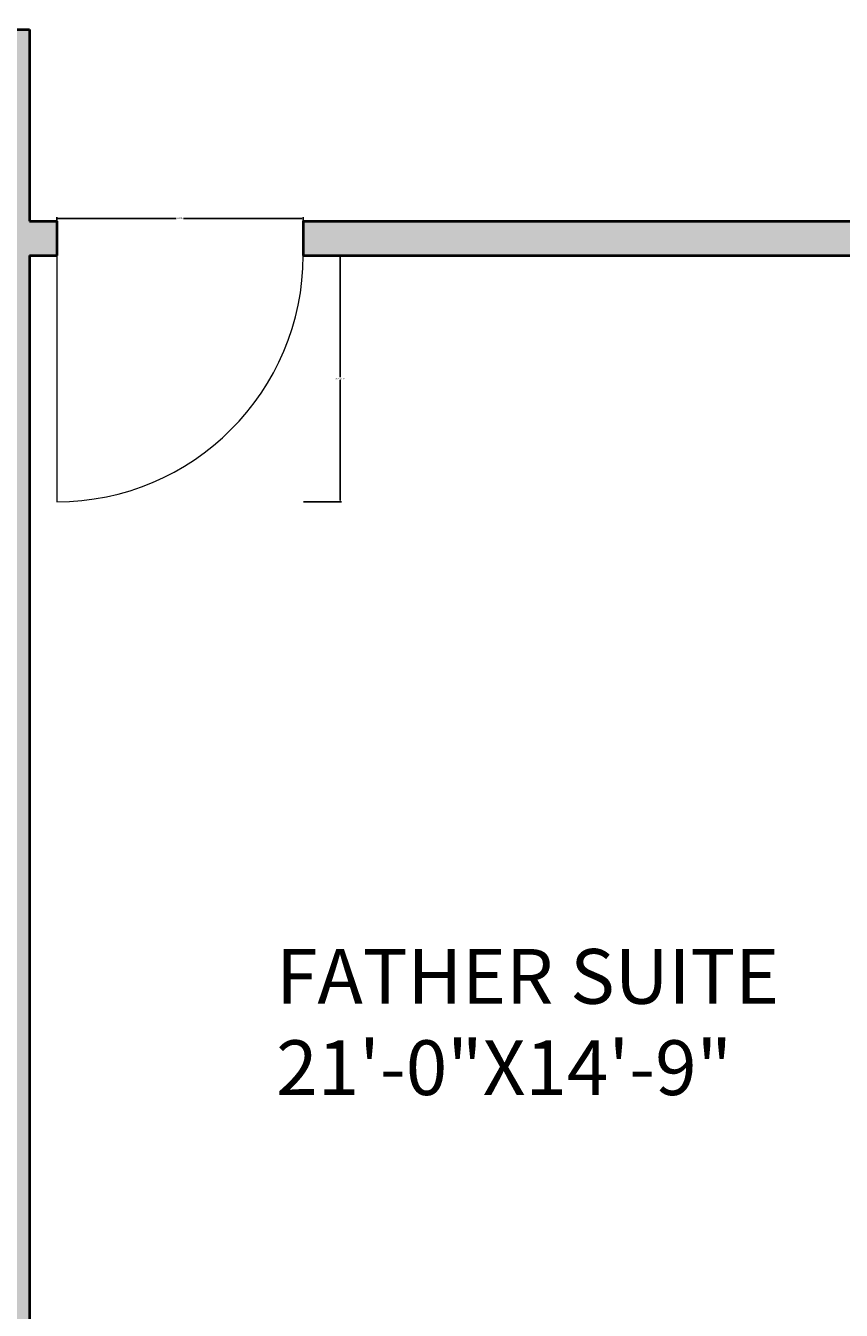
# Model space of a CAD drawing. Units: inches. Extents: x 2330 to 3943, y 1763 to 3461.
# Tile 14 of 40: x 2977 to 3096, y 2547 to 2734. Entities that reach past the tile are written whole.
import ezdxf

# ---------------------------------------------------------------- set-up
doc = ezdxf.new("R2010")
doc.units = ezdxf.units.IN
for name, color, linetype, lineweight in [('A-ANNO-DIMS', 2, 'Continuous', 18), ('A-AREA-IDEN', 7, 'Continuous', 18), ('A-DOOR', 4, 'Continuous', 18), ('A-WALL', 7, 'Continuous', 40), ('A-WALL-PATT', 252, 'Continuous', 13)]:
    doc.layers.add(name, color=color, linetype=linetype, lineweight=lineweight)
doc.styles.get("Standard").update_dxf_attribs({"font": 'arial.ttf'})
doc.dimstyles.get("Standard").update_dxf_attribs({"dimtxt": 0.18, "dimasz": 0.18, "dimexe": 0.18, "dimexo": 0.0625, "dimgap": 0.09, "dimtad": 0, "dimtih": 1, "dimtoh": 1, "dimdec": 4, "dimzin": 0, "dimdsep": 46, "dimtxsty": 'Standard', "dimcen": 0.09, "dimadec": 0, "dimazin": 0, "dimtfac": 1, "dimtdec": 4, "dimtofl": 0, "dimtmove": 0, "dimatfit": 3, "dimfxl": 1, "dimtolj": 1, "dimtzin": 0, "dimarcsym": 0})

# ---------------------------------------------------------------- blocks, each defined once
blk = doc.blocks.new('DOOR-SINGLE-36IN')
blk.add_line((0, 0), (-36, 0))
blk.add_arc((0, 0), 36, 180, 270)
blk = doc.blocks.new('*D27')
at = {"layer": 'A-ANNO-DIMS', "color": 0, "lineweight": -2, "transparency": 16777216}
for p, q in [((3017.72, 2700.65), (3023.24, 2700.65)), ((3023.06, 2700.47), (3023.06, 2682.84)), ((3023.06, 2664.83), (3023.06, 2682.47)), ((3017.72, 2664.65), (3023.24, 2664.65))]:
    blk.add_line(p, q, dxfattribs=at)
at = {"layer": 'A-ANNO-DIMS', "color": 0, "transparency": 16777216}
for points in [[(3023.03, 2700.47), (3023.09, 2700.47), (3023.06, 2700.65)], [(3023.03, 2664.83), (3023.09, 2664.83), (3023.06, 2664.65)]]:
    blk.add_solid(points, dxfattribs=at)
at = {"layer": 'Defpoints', "color": 0, "transparency": 16777216}
for p in [(3017.66, 2700.65), (3023.06, 2700.65), (3017.66, 2664.65)]:
    blk.add_point(p, dxfattribs=at)
at = {"layer": 'A-ANNO-DIMS', "color": 0, "transparency": 16777216, "insert": (3023.06, 2682.65), "char_height": 0.18, "attachment_point": 5}
blk.add_mtext('\\A1;DOOR 36 TYP.', dxfattribs=at)
blk = doc.blocks.new('*D28')
at = {"layer": 'A-ANNO-DIMS', "color": 0, "lineweight": -2, "transparency": 16777216}
for p, q in [((2981.66, 2700.71), (2981.66, 2706.23)), ((2981.84, 2706.05), (2999.13, 2706.05)), ((3017.48, 2706.05), (3000.19, 2706.05)), ((3017.66, 2700.71), (3017.66, 2706.23))]:
    blk.add_line(p, q, dxfattribs=at)
at = {"layer": 'A-ANNO-DIMS', "color": 0, "transparency": 16777216}
for points in [[(2981.84, 2706.08), (2981.84, 2706.02), (2981.66, 2706.05)], [(3017.48, 2706.08), (3017.48, 2706.02), (3017.66, 2706.05)]]:
    blk.add_solid(points, dxfattribs=at)
at = {"layer": 'Defpoints', "color": 0, "transparency": 16777216}
for p in [(2981.66, 2706.05), (2981.66, 2700.65), (3017.66, 2700.65)]:
    blk.add_point(p, dxfattribs=at)
at = {"layer": 'A-ANNO-DIMS', "color": 0, "transparency": 16777216, "insert": (2999.66, 2706.05), "char_height": 0.18, "attachment_point": 5}
blk.add_mtext('\\A1;36 TYP.', dxfattribs=at)

msp = doc.modelspace()

# ---------------------------------------------------------------- hatches: boundary and pattern name
at = {"layer": 'A-WALL-PATT'}
h = msp.add_hatch(color=256, dxfattribs=at)
h.dxf.hatch_style = 1
h.paths.add_polyline_path([(3420.6832, 2705.6524), (3159.6605, 2705.6524), (3159.6605, 2827.6524), (3154.6605, 2827.6524), (3154.6605, 2705.6524), (3017.6605, 2705.6524), (3017.6605, 2700.6524), (3238.6605, 2700.6524), (3238.6605, 2605.6524), (3247.6605, 2605.6524), (3247.6605, 2610.6524), (3243.6605, 2610.6524), (3243.6605, 2700.6524), (3411.2593, 2700.6524, -0.02528333), (3406.9698, 2669.9468), (3415.809, 2668.2528, 0.02988796)])
h = msp.add_hatch(color=256, dxfattribs=at)
h.dxf.hatch_style = 1
h.paths.add_polyline_path([(3203.7816, 2523.6524), (2977.6605, 2523.6524), (2977.6605, 2700.6524), (2981.6605, 2700.6524), (2981.6605, 2705.6524), (2977.6605, 2705.6524), (2977.6605, 2733.6524), (2968.6605, 2733.6524), (2968.6605, 2514.6524), (3023.6605, 2514.6524), (3023.6605, 2510.6524), (3028.6605, 2510.6524), (3028.6605, 2514.6524), (3203.7816, 2514.6524)])

# ---------------------------------------------------------------- linework, layer by layer
at = {"layer": 'A-WALL'}
for p, q in [((2968.6605, 2733.6524), (2977.6605, 2733.6524)), ((2977.6605, 2733.6524), (2977.6605, 2705.6524)), ((2977.6605, 2705.6524), (2981.6605, 2705.6524)), ((2981.6605, 2705.6524), (2981.6605, 2700.6524)), ((3017.6605, 2705.6524), (3017.6605, 2700.6524)), ((3017.6605, 2705.6524), (3154.6605, 2705.6524)), ((2977.6605, 2700.6524), (2981.6605, 2700.6524)), ((2977.6605, 2700.6524), (2977.6605, 2523.6524)), ((3017.6605, 2700.6524), (3238.6605, 2700.6524))]:
    msp.add_line(p, q, dxfattribs=at)

# ---------------------------------------------------------------- block references
at = {"layer": 'A-DOOR', "rotation": 90.00000000000072}
msp.add_blockref('DOOR-SINGLE-36IN', (2981.6605, 2700.6524), dxfattribs=at)

# ---------------------------------------------------------------- texts
at = {"layer": 'A-AREA-IDEN', "insert": (3013.7138, 2599.3322), "char_height": 8, "attachment_point": 1}
msp.add_mtext_dynamic_manual_height_columns('FATHER SUITE\\P21\'-0"X14\'-9"', width=106.674885, gutter_width=12.5, heights=[0], dxfattribs=at)

# ---------------------------------------------------------------- dimensions: what is measured, and where the dimension line sits
at = {"layer": 'A-ANNO-DIMS'}
for base, p1, p2, angle, text, picture, middle in [((2981.6605, 2706.0524), (3017.6605, 2700.6524), (2981.6605, 2700.6524), 180, '<> TYP.', '*D28', (2999.6605, 2706.0524)), ((3023.0605, 2700.6524), (3017.6605, 2664.6524), (3017.6605, 2700.6524), 90, 'DOOR <> TYP.', '*D27', (3023.0605, 2682.6524))]:
    dim = msp.add_linear_dim(base=base, p1=p1, p2=p2, angle=angle, text=text, dimstyle='Standard', override={"dimdec": 0, "dimlfac": 1, "dimrnd": 0, "dimzin": 0, "dimdsep": 46, "dimlunit": 2}, dxfattribs=at)
    dim.commit()
    dim.dimension.update_dxf_attribs({"geometry": picture, "text_midpoint": middle})

doc.saveas('drawing.dxf')
